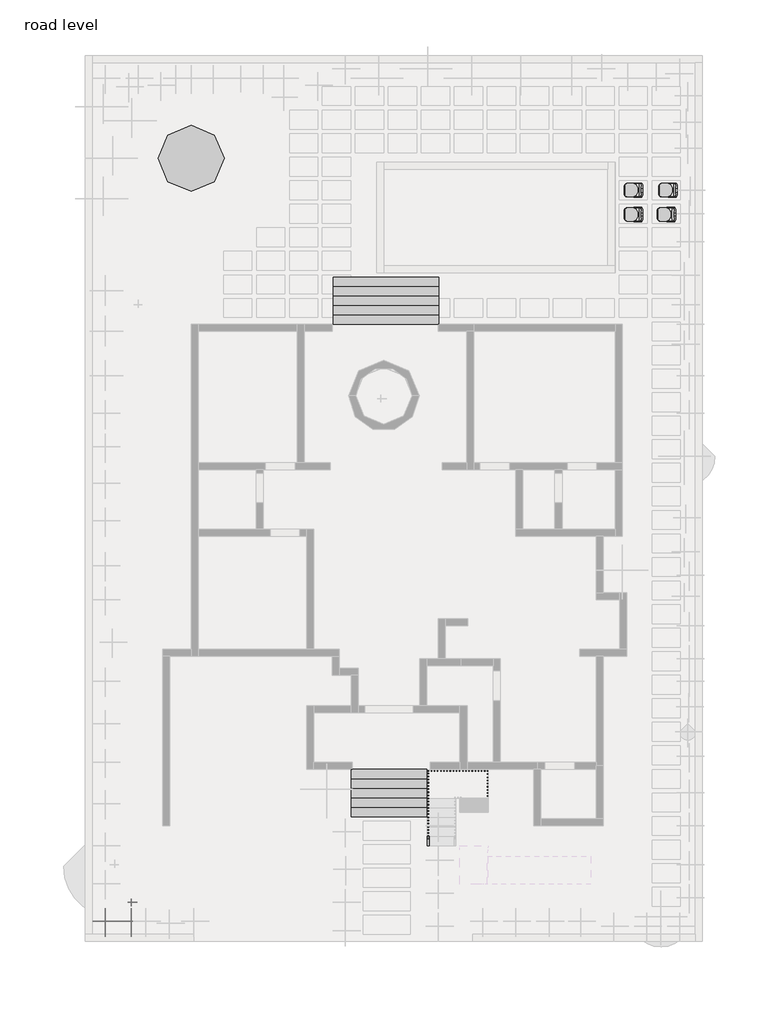
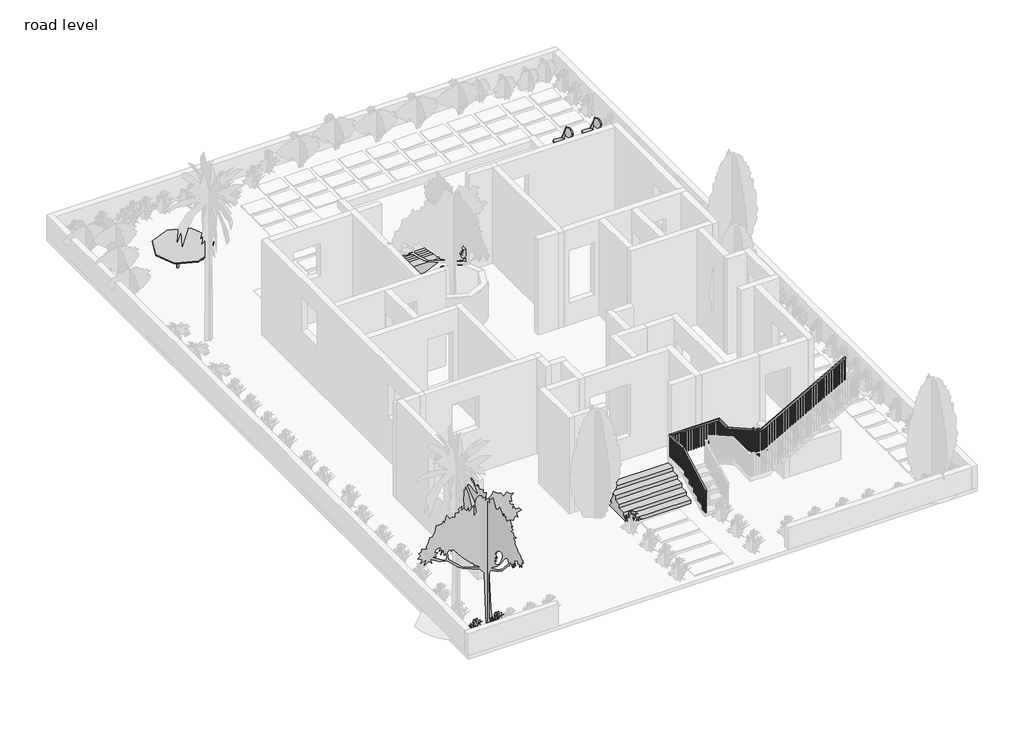
# One storey, part 4 of 5: 7 furniture elements, 3 geographic elements, 1 railing.
"""IFC4 building model written with IfcOpenShell, lengths in millimetres."""

from ifc_helpers import new_model, si_unit, frame, origin, place, context, project, spatial, polyline, outline, extrude, faceted_brep, transform, mapped, element, save
from components import casework_1_casework_1_a8a15752, casework_3_casework_1_715d5e0d, furniture_eb3a3c23, furniture_02b286f5, rpc_plant_tropical_55f6ff97, rpc_tree_tropical_grass_palm_18_ffc4a38a

model = new_model("IFC4")

# Units and contexts
model_context = context("Model", 3, world=origin())
ifc_project = project(units=[si_unit("LENGTHUNIT", "METRE", prefix="MILLI")], contexts=[model_context])

# Site, building, storey
site = spatial("IfcSite", under=ifc_project)
building = spatial("IfcBuilding", under=site)
storey = spatial("IfcBuildingStorey", under=building, Name="road level", Elevation=0.0)

# Furniture
placement = place(None, origin())
casework_1_casework_1_shape = casework_1_casework_1_a8a15752(model_context)
element("IfcFurniture", 1, ObjectType="Casework 1 : Casework 1", at=placement, inside=storey, context=model_context, shape_type="MappedRepresentation", body=[
    mapped(casework_1_casework_1_shape, transform((0.0, 0.0, 0.0), x_axis=(1.0, 0.0, 0.0), y_axis=(0.0, 1.0, 0.0), z_axis=(0.0, 0.0, 1.0))),
])
casework_3_casework_1_shape = casework_3_casework_1_715d5e0d(model_context)
element("IfcFurniture", 2, ObjectType="Casework 3 : Casework 1", at=placement, inside=storey, context=model_context, shape_type="MappedRepresentation", body=[
    mapped(casework_3_casework_1_shape, transform((0.0, 0.0, 0.0), x_axis=(1.0, 0.0, 0.0), y_axis=(0.0, 1.0, 0.0), z_axis=(0.0, 0.0, 1.0))),
])
furniture_shape = furniture_eb3a3c23(model_context)
element("IfcFurniture", 3, ObjectType="Seating-Auditorium : 18\" x 24\" x 30\"", at=placement, inside=storey, context=model_context, shape_type="MappedRepresentation", body=[
    mapped(furniture_shape, transform((13048.714907, 18716.9628198, 50.8), x_axis=(0.0, 1.0, 0.0), y_axis=(-1.0, 0.0, 0.0), z_axis=(0.0, 0.0, 1.0))),
])
element("IfcFurniture", 4, ObjectType="Seating-Auditorium : 18\" x 24\" x 30\"", at=placement, inside=storey, context=model_context, shape_type="MappedRepresentation", body=[
    mapped(furniture_shape, transform((13048.714907, 17929.5628198, 50.8), x_axis=(0.0, 1.0, 0.0), y_axis=(-1.0, 0.0, 0.0), z_axis=(0.0, 0.0, 1.0))),
])
element("IfcFurniture", 5, ObjectType="Seating-Auditorium : 18\" x 24\" x 30\"", at=placement, inside=storey, context=model_context, shape_type="MappedRepresentation", body=[
    mapped(furniture_shape, transform((14115.514907, 17929.5628198, 50.8), x_axis=(0.0, 1.0, 0.0), y_axis=(-1.0, 0.0, 0.0), z_axis=(0.0, 0.0, 1.0))),
])
element("IfcFurniture", 6, ObjectType="Seating-Auditorium : 18\" x 24\" x 30\"", at=placement, inside=storey, context=model_context, shape_type="MappedRepresentation", body=[
    mapped(furniture_shape, transform((14166.314907, 18716.9628198, 50.8), x_axis=(0.0, 1.0, 0.0), y_axis=(-1.0, 0.0, 0.0), z_axis=(0.0, 0.0, 1.0))),
])
furniture_2_shape = furniture_02b286f5(model_context)
element("IfcFurniture", 7, ObjectType="Table-Dining Round : 84\" Diameter", at=placement, inside=storey, context=model_context, shape_type="MappedRepresentation", body=[
    mapped(furniture_2_shape, transform((-1573.2306847, 20091.2693772, 0.0), x_axis=(1.0, 0.0, 0.0), y_axis=(0.0, 1.0, 0.0), z_axis=(0.0, 0.0, 1.0))),
])

# Geographic elements
rpc_plant_tropical_shape = rpc_plant_tropical_55f6ff97(model_context)
element("IfcGeographicElement", 8, ObjectType="RPC Plant - Tropical", at=placement, inside=storey, context=model_context, shape_type="MappedRepresentation", body=[
    mapped(rpc_plant_tropical_shape, transform((-4250.8487175, -4782.4093114, 0.0), x_axis=(1.0, 0.0, 0.0), y_axis=(0.0, 1.0, 0.0), z_axis=(0.0, 0.0, 1.0))),
])
element("IfcGeographicElement", 9, ObjectType="RPC Plant - Tropical", at=placement, inside=storey, context=model_context, shape_type="MappedRepresentation", body=[
    mapped(rpc_plant_tropical_shape, transform((-3412.6487175, -4782.4093114, 0.0), x_axis=(1.0, 0.0, 0.0), y_axis=(0.0, 1.0, 0.0), z_axis=(0.0, 0.0, 1.0))),
])
rpc_tree_tropical_grass_palm_18_shape = rpc_tree_tropical_grass_palm_18_ffc4a38a(model_context)
element("IfcGeographicElement", 10, ObjectType="RPC Tree - Tropical : Grass Palm - 18'", at=placement, inside=storey, context=model_context, shape_type="MappedRepresentation", body=[
    mapped(rpc_tree_tropical_grass_palm_18_shape, transform((-3412.6487175, -4172.8093114, 0.0), x_axis=(1.0, 0.0, 0.0), y_axis=(0.0, 1.0, 0.0), z_axis=(0.0, 0.0, 1.0))),
])

# Railing
element("IfcRailing", 11, ObjectType="Handrail - Rectangular", at=placement, inside=storey, context=model_context, shape_type="SolidModel", body=[
    faceted_brep([(6178.0083823, -2332.334977, 1085.85), (6178.0083823, -2332.334977, 1027.5647478), (6228.8083823, -2332.334977, 1027.5647478), (6228.8083823, -2332.334977, 1085.85), (6178.0083823, -808.334977, 1943.1), (6178.0083823, -795.0278619, 1892.3), (6228.8083823, -795.0278619, 1892.3), (6228.8083823, -808.334977, 1943.1), (6178.0083823, 106.065023, 1943.1), (6178.0083823, 106.065023, 1892.3), (6228.8083823, 55.265023, 1892.3), (6228.8083823, 55.265023, 1943.1), (8143.1297505, 106.065023, 1943.1), (8143.1297505, 106.065023, 1892.3), (8092.3297505, 55.265023, 1892.3), (8092.3297505, 55.265023, 1943.1), (8143.1297505, -503.534977, 1943.1), (8143.1297505, -516.842092, 1892.3), (8092.3297505, -516.842092, 1892.3), (8092.3297505, -503.534977, 1943.1), (8143.1297505, -808.334977, 2114.55), (8143.1297505, -833.2402479, 2070.2739627), (8092.3297505, -833.2402479, 2070.2739627), (8092.3297505, -808.334977, 2114.55), (8143.1297505, -2229.3239999, 2913.8563254), (8143.1297505, -2280.1239999, 2884.1460732), (8092.3297505, -2280.1239999, 2884.1460732), (8092.3297505, -2229.3239999, 2913.8563254), (8143.1297505, -2229.3239999, 2971.8), (8143.1297505, -2280.1239999, 2921.0), (8092.3297505, -2280.1239999, 2921.0), (8092.3297505, -2229.3239999, 2971.8), (8143.1297505, -2332.334977, 2971.8), (8143.1297505, -2332.334977, 2921.0), (8092.3297505, -2329.5130228, 2921.0), (8092.3297505, -2329.5130228, 2971.8), (8131.7203808, -2434.7121604, 2971.8), (8131.7203808, -2434.7121604, 2921.0), (8081.232937, -2429.0856146, 2921.0), (8081.232937, -2429.0856146, 2971.8), (8113.1386293, -2601.4476967, 2971.8), (8107.5120834, -2651.9351405, 2921.0), (8057.0246396, -2646.3085946, 2921.0), (8062.6511855, -2595.8211508, 2971.8), (8113.1386293, -2601.4476967, 3184.4317867), (8107.5120834, -2651.9351405, 3133.6317867), (8057.0246396, -2646.3085946, 3133.6317867), (8062.6511855, -2595.8211508, 3184.4317867), (8105.0297505, -2674.2093114, 3184.4317867), (8105.0297505, -2674.2093114, 3133.6317867), (8048.2538809, -2725.0093114, 3133.6317867), (8048.2538809, -2725.0093114, 3184.4317867), (8178.2418157, -2674.2093114, 3184.4317867), (8191.5489308, -2674.2093114, 3133.6317867), (8191.5489308, -2725.0093114, 3133.6317867), (8178.2418157, -2725.0093114, 3184.4317867), (11457.8297505, -2674.2093114, 5029.2), (11457.8297505, -2725.0093114, 5029.2), (11457.8297505, -2725.0093114, 4970.9147478), (11457.8297505, -2674.2093114, 4970.9147478)], [[[0, 1, 2, 3]], [[1, 0, 4, 5]], [[2, 1, 5, 6]], [[3, 2, 6, 7]], [[0, 3, 7, 4]], [[5, 4, 8, 9]], [[6, 5, 9, 10]], [[7, 6, 10, 11]], [[4, 7, 11, 8]], [[9, 8, 12, 13]], [[10, 9, 13, 14]], [[11, 10, 14, 15]], [[8, 11, 15, 12]], [[13, 12, 16, 17]], [[14, 13, 17, 18]], [[15, 14, 18, 19]], [[12, 15, 19, 16]], [[17, 16, 20, 21]], [[18, 17, 21, 22]], [[19, 18, 22, 23]], [[16, 19, 23, 20]], [[21, 20, 24, 25]], [[22, 21, 25, 26]], [[23, 22, 26, 27]], [[20, 23, 27, 24]], [[25, 24, 28, 29]], [[26, 25, 29, 30]], [[27, 26, 30, 31]], [[24, 27, 31, 28]], [[29, 28, 32, 33]], [[30, 29, 33, 34]], [[31, 30, 34, 35]], [[28, 31, 35, 32]], [[33, 32, 36, 37]], [[34, 33, 37, 38]], [[35, 34, 38, 39]], [[32, 35, 39, 36]], [[37, 36, 40, 41]], [[38, 37, 41, 42]], [[39, 38, 42, 43]], [[36, 39, 43, 40]], [[41, 40, 44, 45]], [[42, 41, 45, 46]], [[43, 42, 46, 47]], [[40, 43, 47, 44]], [[45, 44, 48, 49]], [[46, 45, 49, 50]], [[47, 46, 50, 51]], [[44, 47, 51, 48]], [[49, 48, 52, 53]], [[50, 49, 53, 54]], [[51, 50, 54, 55]], [[48, 51, 55, 52]], [[56, 57, 58, 59]], [[53, 52, 56, 59]], [[54, 53, 59, 58]], [[55, 54, 58, 57]], [[52, 55, 57, 56]]]),
    extrude(outline(polyline([(4949.588722, 11419.9168157), (3943.35, 11419.9168157), (3943.35, 11438.9668157), (4960.304347, 11438.9668157), (4949.588722, 11419.9168157)])), frame((0.0, -2709.1343114, 0.0), z_axis=(0.0, 1.0, 0.0), x_axis=(0.0, 0.0, 1.0)), (0.0, 0.0, 1.0), 19.05),
    extrude(outline(polyline([(4892.438722, 11318.3168157), (3943.35, 11318.3168157), (3943.35, 11337.3668157), (4903.154347, 11337.3668157), (4892.438722, 11318.3168157)])), frame((0.0, -2709.1343114, 0.0), z_axis=(0.0, 1.0, 0.0), x_axis=(0.0, 0.0, 1.0)), (0.0, 0.0, 1.0), 19.05),
    extrude(outline(polyline([(4835.288722, 11216.7168157), (3943.35, 11216.7168157), (3943.35, 11235.7668157), (4846.004347, 11235.7668157), (4835.288722, 11216.7168157)])), frame((0.0, -2709.1343114, 0.0), z_axis=(0.0, 1.0, 0.0), x_axis=(0.0, 0.0, 1.0)), (0.0, 0.0, 1.0), 19.05),
    extrude(outline(polyline([(4778.138722, 11115.1168157), (3771.9, 11115.1168157), (3771.9, 11134.1668157), (4788.854347, 11134.1668157), (4778.138722, 11115.1168157)])), frame((0.0, -2709.1343114, 0.0), z_axis=(0.0, 1.0, 0.0), x_axis=(0.0, 0.0, 1.0)), (0.0, 0.0, 1.0), 19.05),
    extrude(outline(polyline([(4720.988722, 11013.5168157), (3771.9, 11013.5168157), (3771.9, 11032.5668157), (4731.704347, 11032.5668157), (4720.988722, 11013.5168157)])), frame((0.0, -2709.1343114, 0.0), z_axis=(0.0, 1.0, 0.0), x_axis=(0.0, 0.0, 1.0)), (0.0, 0.0, 1.0), 19.05),
    extrude(outline(polyline([(4663.838722, 10911.9168157), (3771.9, 10911.9168157), (3771.9, 10930.9668157), (4674.554347, 10930.9668157), (4663.838722, 10911.9168157)])), frame((0.0, -2709.1343114, 0.0), z_axis=(0.0, 1.0, 0.0), x_axis=(0.0, 0.0, 1.0)), (0.0, 0.0, 1.0), 19.05),
    extrude(outline(polyline([(4606.688722, 10810.3168157), (3600.45, 10810.3168157), (3600.45, 10829.3668157), (4617.404347, 10829.3668157), (4606.688722, 10810.3168157)])), frame((0.0, -2709.1343114, 0.0), z_axis=(0.0, 1.0, 0.0), x_axis=(0.0, 0.0, 1.0)), (0.0, 0.0, 1.0), 19.05),
    extrude(outline(polyline([(4549.538722, 10708.7168157), (3600.45, 10708.7168157), (3600.45, 10727.7668157), (4560.254347, 10727.7668157), (4549.538722, 10708.7168157)])), frame((0.0, -2709.1343114, 0.0), z_axis=(0.0, 1.0, 0.0), x_axis=(0.0, 0.0, 1.0)), (0.0, 0.0, 1.0), 19.05),
    extrude(outline(polyline([(4492.388722, 10607.1168157), (3600.45, 10607.1168157), (3600.45, 10626.1668157), (4503.104347, 10626.1668157), (4492.388722, 10607.1168157)])), frame((0.0, -2709.1343114, 0.0), z_axis=(0.0, 1.0, 0.0), x_axis=(0.0, 0.0, 1.0)), (0.0, 0.0, 1.0), 19.05),
    extrude(outline(polyline([(4435.238722, 10505.5168157), (3429.0, 10505.5168157), (3429.0, 10524.5668157), (4445.954347, 10524.5668157), (4435.238722, 10505.5168157)])), frame((0.0, -2709.1343114, 0.0), z_axis=(0.0, 1.0, 0.0), x_axis=(0.0, 0.0, 1.0)), (0.0, 0.0, 1.0), 19.05),
    extrude(outline(polyline([(4378.088722, 10403.9168157), (3429.0, 10403.9168157), (3429.0, 10422.9668157), (4388.804347, 10422.9668157), (4378.088722, 10403.9168157)])), frame((0.0, -2709.1343114, 0.0), z_axis=(0.0, 1.0, 0.0), x_axis=(0.0, 0.0, 1.0)), (0.0, 0.0, 1.0), 19.05),
    extrude(outline(polyline([(4320.938722, 10302.3168157), (3429.0, 10302.3168157), (3429.0, 10321.3668157), (4331.654347, 10321.3668157), (4320.938722, 10302.3168157)])), frame((0.0, -2709.1343114, 0.0), z_axis=(0.0, 1.0, 0.0), x_axis=(0.0, 0.0, 1.0)), (0.0, 0.0, 1.0), 19.05),
    extrude(outline(polyline([(4263.788722, 10200.7168157), (3257.55, 10200.7168157), (3257.55, 10219.7668157), (4274.504347, 10219.7668157), (4263.788722, 10200.7168157)])), frame((0.0, -2709.1343114, 0.0), z_axis=(0.0, 1.0, 0.0), x_axis=(0.0, 0.0, 1.0)), (0.0, 0.0, 1.0), 19.05),
    extrude(outline(polyline([(4206.638722, 10099.1168157), (3257.55, 10099.1168157), (3257.55, 10118.1668157), (4217.354347, 10118.1668157), (4206.638722, 10099.1168157)])), frame((0.0, -2709.1343114, 0.0), z_axis=(0.0, 1.0, 0.0), x_axis=(0.0, 0.0, 1.0)), (0.0, 0.0, 1.0), 19.05),
    extrude(outline(polyline([(4149.488722, 9997.5168157), (3257.55, 9997.5168157), (3257.55, 10016.5668157), (4160.204347, 10016.5668157), (4149.488722, 9997.5168157)])), frame((0.0, -2709.1343114, 0.0), z_axis=(0.0, 1.0, 0.0), x_axis=(0.0, 0.0, 1.0)), (0.0, 0.0, 1.0), 19.05),
    extrude(outline(polyline([(4092.338722, 9895.9168157), (3086.1, 9895.9168157), (3086.1, 9914.9668157), (4103.054347, 9914.9668157), (4092.338722, 9895.9168157)])), frame((0.0, -2709.1343114, 0.0), z_axis=(0.0, 1.0, 0.0), x_axis=(0.0, 0.0, 1.0)), (0.0, 0.0, 1.0), 19.05),
    extrude(outline(polyline([(4035.188722, 9794.3168157), (3086.1, 9794.3168157), (3086.1, 9813.3668157), (4045.904347, 9813.3668157), (4035.188722, 9794.3168157)])), frame((0.0, -2709.1343114, 0.0), z_axis=(0.0, 1.0, 0.0), x_axis=(0.0, 0.0, 1.0)), (0.0, 0.0, 1.0), 19.05),
    extrude(outline(polyline([(3978.038722, 9692.7168157), (3086.1, 9692.7168157), (3086.1, 9711.7668157), (3988.754347, 9711.7668157), (3978.038722, 9692.7168157)])), frame((0.0, -2709.1343114, 0.0), z_axis=(0.0, 1.0, 0.0), x_axis=(0.0, 0.0, 1.0)), (0.0, 0.0, 1.0), 19.05),
    extrude(outline(polyline([(3920.888722, 9591.1168157), (2914.65, 9591.1168157), (2914.65, 9610.1668157), (3931.604347, 9610.1668157), (3920.888722, 9591.1168157)])), frame((0.0, -2709.1343114, 0.0), z_axis=(0.0, 1.0, 0.0), x_axis=(0.0, 0.0, 1.0)), (0.0, 0.0, 1.0), 19.05),
    extrude(outline(polyline([(3863.738722, 9489.5168157), (2914.65, 9489.5168157), (2914.65, 9508.5668157), (3874.454347, 9508.5668157), (3863.738722, 9489.5168157)])), frame((0.0, -2709.1343114, 0.0), z_axis=(0.0, 1.0, 0.0), x_axis=(0.0, 0.0, 1.0)), (0.0, 0.0, 1.0), 19.05),
    extrude(outline(polyline([(3806.588722, 9387.9168157), (2914.65, 9387.9168157), (2914.65, 9406.9668157), (3817.304347, 9406.9668157), (3806.588722, 9387.9168157)])), frame((0.0, -2709.1343114, 0.0), z_axis=(0.0, 1.0, 0.0), x_axis=(0.0, 0.0, 1.0)), (0.0, 0.0, 1.0), 19.05),
    extrude(outline(polyline([(3749.438722, 9286.3168157), (2743.2, 9286.3168157), (2743.2, 9305.3668157), (3760.154347, 9305.3668157), (3749.438722, 9286.3168157)])), frame((0.0, -2709.1343114, 0.0), z_axis=(0.0, 1.0, 0.0), x_axis=(0.0, 0.0, 1.0)), (0.0, 0.0, 1.0), 19.05),
    extrude(outline(polyline([(3692.288722, 9184.7168157), (2743.2, 9184.7168157), (2743.2, 9203.7668157), (3703.004347, 9203.7668157), (3692.288722, 9184.7168157)])), frame((0.0, -2709.1343114, 0.0), z_axis=(0.0, 1.0, 0.0), x_axis=(0.0, 0.0, 1.0)), (0.0, 0.0, 1.0), 19.05),
    extrude(outline(polyline([(3635.138722, 9083.1168157), (2743.2, 9083.1168157), (2743.2, 9102.1668157), (3645.854347, 9102.1668157), (3635.138722, 9083.1168157)])), frame((0.0, -2709.1343114, 0.0), z_axis=(0.0, 1.0, 0.0), x_axis=(0.0, 0.0, 1.0)), (0.0, 0.0, 1.0), 19.05),
    extrude(outline(polyline([(3577.988722, 8981.5168157), (2571.75, 8981.5168157), (2571.75, 9000.5668157), (3588.704347, 9000.5668157), (3577.988722, 8981.5168157)])), frame((0.0, -2709.1343114, 0.0), z_axis=(0.0, 1.0, 0.0), x_axis=(0.0, 0.0, 1.0)), (0.0, 0.0, 1.0), 19.05),
    extrude(outline(polyline([(3520.838722, 8879.9168157), (2571.75, 8879.9168157), (2571.75, 8898.9668157), (3531.554347, 8898.9668157), (3520.838722, 8879.9168157)])), frame((0.0, -2709.1343114, 0.0), z_axis=(0.0, 1.0, 0.0), x_axis=(0.0, 0.0, 1.0)), (0.0, 0.0, 1.0), 19.05),
    extrude(outline(polyline([(3463.688722, 8778.3168157), (2571.75, 8778.3168157), (2571.75, 8797.3668157), (3474.404347, 8797.3668157), (3463.688722, 8778.3168157)])), frame((0.0, -2709.1343114, 0.0), z_axis=(0.0, 1.0, 0.0), x_axis=(0.0, 0.0, 1.0)), (0.0, 0.0, 1.0), 19.05),
    extrude(outline(polyline([(3406.538722, 8676.7168157), (2400.3, 8676.7168157), (2400.3, 8695.7668157), (3417.254347, 8695.7668157), (3406.538722, 8676.7168157)])), frame((0.0, -2709.1343114, 0.0), z_axis=(0.0, 1.0, 0.0), x_axis=(0.0, 0.0, 1.0)), (0.0, 0.0, 1.0), 19.05),
    extrude(outline(polyline([(3349.388722, 8575.1168157), (2400.3, 8575.1168157), (2400.3, 8594.1668157), (3360.104347, 8594.1668157), (3349.388722, 8575.1168157)])), frame((0.0, -2709.1343114, 0.0), z_axis=(0.0, 1.0, 0.0), x_axis=(0.0, 0.0, 1.0)), (0.0, 0.0, 1.0), 19.05),
    extrude(outline(polyline([(3292.238722, 8473.5168157), (2400.3, 8473.5168157), (2400.3, 8492.5668157), (3302.954347, 8492.5668157), (3292.238722, 8473.5168157)])), frame((0.0, -2709.1343114, 0.0), z_axis=(0.0, 1.0, 0.0), x_axis=(0.0, 0.0, 1.0)), (0.0, 0.0, 1.0), 19.05),
    extrude(outline(polyline([(3235.088722, 8371.9168157), (2228.85, 8371.9168157), (2228.85, 8390.9668157), (3245.804347, 8390.9668157), (3235.088722, 8371.9168157)])), frame((0.0, -2709.1343114, 0.0), z_axis=(0.0, 1.0, 0.0), x_axis=(0.0, 0.0, 1.0)), (0.0, 0.0, 1.0), 19.05),
    extrude(outline(polyline([(3177.938722, 8270.3168157), (2228.85, 8270.3168157), (2228.85, 8289.3668157), (3188.654347, 8289.3668157), (3177.938722, 8270.3168157)])), frame((0.0, -2709.1343114, 0.0), z_axis=(0.0, 1.0, 0.0), x_axis=(0.0, 0.0, 1.0)), (0.0, 0.0, 1.0), 19.05),
    extrude(outline(polyline([(3120.788722, 8168.7168157), (2228.85, 8168.7168157), (2228.85, 8187.7668157), (3131.504347, 8187.7668157), (3120.788722, 8168.7168157)])), frame((0.0, -2709.1343114, 0.0), z_axis=(0.0, 1.0, 0.0), x_axis=(0.0, 0.0, 1.0)), (0.0, 0.0, 1.0), 19.05),
    extrude(outline(polyline([(8094.4918486, -2625.4372443), (8092.381894, -2644.3700358), (8073.4491025, -2642.2600811), (8075.5590572, -2623.3272896), (8094.4918486, -2625.4372443)])), frame((0.0, 0.0, 2057.4), z_axis=(0.0, 0.0, 1.0), x_axis=(1.0, 0.0, 0.0)), (0.0, 0.0, 1.0), 1076.2317867),
    extrude(outline(polyline([(8105.7449403, -2524.4623567), (8103.6349856, -2543.3951481), (8084.7021942, -2541.2851935), (8086.8121489, -2522.352402), (8105.7449403, -2524.4623567)])), frame((0.0, 0.0, 2057.4), z_axis=(0.0, 0.0, 1.0), x_axis=(1.0, 0.0, 0.0)), (0.0, 0.0, 1.0), 863.6),
    extrude(outline(polyline([(8116.9980319, -2423.4874691), (8114.8880773, -2442.4202605), (8095.9552858, -2440.3103059), (8098.0652405, -2421.3775144), (8116.9980319, -2423.4874691)])), frame((0.0, 0.0, 2057.4), z_axis=(0.0, 0.0, 1.0), x_axis=(1.0, 0.0, 0.0)), (0.0, 0.0, 1.0), 863.6),
    extrude(outline(polyline([(8127.2547505, -2221.209977), (8127.2547505, -2240.259977), (8108.2047505, -2240.259977), (8108.2047505, -2221.209977), (8127.2547505, -2221.209977)])), frame((0.0, 0.0, 1885.95), z_axis=(0.0, 0.0, 1.0), x_axis=(1.0, 0.0, 0.0)), (0.0, 0.0, 1.0), 1035.05),
    extrude(outline(polyline([(-2119.609977, 2793.8569353), (-2119.609977, 1885.95), (-2138.659977, 1885.95), (-2138.659977, 2804.5725603), (-2119.609977, 2793.8569353)])), frame((8108.2047505, 0.0, 0.0), z_axis=(1.0, 0.0, 0.0), x_axis=(0.0, 1.0, 0.0)), (0.0, 0.0, 1.0), 19.05),
    extrude(outline(polyline([(-2018.009977, 2736.7069353), (-2018.009977, 1885.95), (-2037.059977, 1885.95), (-2037.059977, 2747.4225603), (-2018.009977, 2736.7069353)])), frame((8108.2047505, 0.0, 0.0), z_axis=(1.0, 0.0, 0.0), x_axis=(0.0, 1.0, 0.0)), (0.0, 0.0, 1.0), 19.05),
    extrude(outline(polyline([(-1916.409977, 2679.5569353), (-1916.409977, 1714.5), (-1935.459977, 1714.5), (-1935.459977, 2690.2725603), (-1916.409977, 2679.5569353)])), frame((8108.2047505, 0.0, 0.0), z_axis=(1.0, 0.0, 0.0), x_axis=(0.0, 1.0, 0.0)), (0.0, 0.0, 1.0), 19.05),
    extrude(outline(polyline([(-1814.809977, 2622.4069353), (-1814.809977, 1714.5), (-1833.859977, 1714.5), (-1833.859977, 2633.1225603), (-1814.809977, 2622.4069353)])), frame((8108.2047505, 0.0, 0.0), z_axis=(1.0, 0.0, 0.0), x_axis=(0.0, 1.0, 0.0)), (0.0, 0.0, 1.0), 19.05),
    extrude(outline(polyline([(-1713.209977, 2565.2569353), (-1713.209977, 1714.5), (-1732.259977, 1714.5), (-1732.259977, 2575.9725603), (-1713.209977, 2565.2569353)])), frame((8108.2047505, 0.0, 0.0), z_axis=(1.0, 0.0, 0.0), x_axis=(0.0, 1.0, 0.0)), (0.0, 0.0, 1.0), 19.05),
    extrude(outline(polyline([(-1611.609977, 2508.1069353), (-1611.609977, 1543.05), (-1630.659977, 1543.05), (-1630.659977, 2518.8225603), (-1611.609977, 2508.1069353)])), frame((8108.2047505, 0.0, 0.0), z_axis=(1.0, 0.0, 0.0), x_axis=(0.0, 1.0, 0.0)), (0.0, 0.0, 1.0), 19.05),
    extrude(outline(polyline([(-1510.009977, 2450.9569353), (-1510.009977, 1543.05), (-1529.059977, 1543.05), (-1529.059977, 2461.6725603), (-1510.009977, 2450.9569353)])), frame((8108.2047505, 0.0, 0.0), z_axis=(1.0, 0.0, 0.0), x_axis=(0.0, 1.0, 0.0)), (0.0, 0.0, 1.0), 19.05),
    extrude(outline(polyline([(-1408.409977, 2393.8069353), (-1408.409977, 1543.05), (-1427.459977, 1543.05), (-1427.459977, 2404.5225603), (-1408.409977, 2393.8069353)])), frame((8108.2047505, 0.0, 0.0), z_axis=(1.0, 0.0, 0.0), x_axis=(0.0, 1.0, 0.0)), (0.0, 0.0, 1.0), 19.05),
    extrude(outline(polyline([(-1306.809977, 2336.6569353), (-1306.809977, 1371.6), (-1325.859977, 1371.6), (-1325.859977, 2347.3725603), (-1306.809977, 2336.6569353)])), frame((8108.2047505, 0.0, 0.0), z_axis=(1.0, 0.0, 0.0), x_axis=(0.0, 1.0, 0.0)), (0.0, 0.0, 1.0), 19.05),
    extrude(outline(polyline([(-1205.209977, 2279.5069353), (-1205.209977, 1371.6), (-1224.259977, 1371.6), (-1224.259977, 2290.2225603), (-1205.209977, 2279.5069353)])), frame((8108.2047505, 0.0, 0.0), z_axis=(1.0, 0.0, 0.0), x_axis=(0.0, 1.0, 0.0)), (0.0, 0.0, 1.0), 19.05),
    extrude(outline(polyline([(-1103.609977, 2222.3569353), (-1103.609977, 1371.6), (-1122.659977, 1371.6), (-1122.659977, 2233.0725603), (-1103.609977, 2222.3569353)])), frame((8108.2047505, 0.0, 0.0), z_axis=(1.0, 0.0, 0.0), x_axis=(0.0, 1.0, 0.0)), (0.0, 0.0, 1.0), 19.05),
    extrude(outline(polyline([(-1002.009977, 2165.2069353), (-1002.009977, 1200.15), (-1021.059977, 1200.15), (-1021.059977, 2175.9225603), (-1002.009977, 2165.2069353)])), frame((8108.2047505, 0.0, 0.0), z_axis=(1.0, 0.0, 0.0), x_axis=(0.0, 1.0, 0.0)), (0.0, 0.0, 1.0), 19.05),
    extrude(outline(polyline([(-900.409977, 2108.0569353), (-900.409977, 1200.15), (-919.459977, 1200.15), (-919.459977, 2118.7725603), (-900.409977, 2108.0569353)])), frame((8108.2047505, 0.0, 0.0), z_axis=(1.0, 0.0, 0.0), x_axis=(0.0, 1.0, 0.0)), (0.0, 0.0, 1.0), 19.05),
    extrude(outline(polyline([(-722.609977, 2008.0444353), (-722.609977, 1028.7), (-741.659977, 1028.7), (-741.659977, 2018.7600603), (-722.609977, 2008.0444353)])), frame((8108.2047505, 0.0, 0.0), z_axis=(1.0, 0.0, 0.0), x_axis=(0.0, 1.0, 0.0)), (0.0, 0.0, 1.0), 19.05),
    extrude(outline(polyline([(-621.009977, 1950.8944353), (-621.009977, 1028.7), (-640.059977, 1028.7), (-640.059977, 1961.6100603), (-621.009977, 1950.8944353)])), frame((8108.2047505, 0.0, 0.0), z_axis=(1.0, 0.0, 0.0), x_axis=(0.0, 1.0, 0.0)), (0.0, 0.0, 1.0), 19.05),
    extrude(outline(polyline([(-519.409977, 1893.7444353), (-519.409977, 1028.7), (-538.459977, 1028.7), (-538.459977, 1904.4600603), (-519.409977, 1893.7444353)])), frame((8108.2047505, 0.0, 0.0), z_axis=(1.0, 0.0, 0.0), x_axis=(0.0, 1.0, 0.0)), (0.0, 0.0, 1.0), 19.05),
    extrude(outline(polyline([(8127.2547505, -417.809977), (8127.2547505, -436.859977), (8108.2047505, -436.859977), (8108.2047505, -417.809977), (8127.2547505, -417.809977)])), frame((0.0, 0.0, 1028.7), z_axis=(0.0, 0.0, 1.0), x_axis=(1.0, 0.0, 0.0)), (0.0, 0.0, 1.0), 863.6),
    extrude(outline(polyline([(8127.2547505, -316.209977), (8127.2547505, -335.259977), (8108.2047505, -335.259977), (8108.2047505, -316.209977), (8127.2547505, -316.209977)])), frame((0.0, 0.0, 1028.7), z_axis=(0.0, 0.0, 1.0), x_axis=(1.0, 0.0, 0.0)), (0.0, 0.0, 1.0), 863.6),
    extrude(outline(polyline([(8127.2547505, -214.609977), (8127.2547505, -233.659977), (8108.2047505, -233.659977), (8108.2047505, -214.609977), (8127.2547505, -214.609977)])), frame((0.0, 0.0, 1028.7), z_axis=(0.0, 0.0, 1.0), x_axis=(1.0, 0.0, 0.0)), (0.0, 0.0, 1.0), 863.6),
    extrude(outline(polyline([(8127.2547505, -113.009977), (8127.2547505, -132.059977), (8108.2047505, -132.059977), (8108.2047505, -113.009977), (8127.2547505, -113.009977)])), frame((0.0, 0.0, 1028.7), z_axis=(0.0, 0.0, 1.0), x_axis=(1.0, 0.0, 0.0)), (0.0, 0.0, 1.0), 863.6),
    extrude(outline(polyline([(8127.2547505, -11.409977), (8127.2547505, -30.459977), (8108.2047505, -30.459977), (8108.2047505, -11.409977), (8127.2547505, -11.409977)])), frame((0.0, 0.0, 1028.7), z_axis=(0.0, 0.0, 1.0), x_axis=(1.0, 0.0, 0.0)), (0.0, 0.0, 1.0), 863.6),
    extrude(outline(polyline([(8022.6833823, 90.190023), (8041.7333823, 90.190023), (8041.7333823, 71.140023), (8022.6833823, 71.140023), (8022.6833823, 90.190023)])), frame((0.0, 0.0, 1028.7), z_axis=(0.0, 0.0, 1.0), x_axis=(1.0, 0.0, 0.0)), (0.0, 0.0, 1.0), 863.6),
    extrude(outline(polyline([(7921.0833823, 90.190023), (7940.1333823, 90.190023), (7940.1333823, 71.140023), (7921.0833823, 71.140023), (7921.0833823, 90.190023)])), frame((0.0, 0.0, 1028.7), z_axis=(0.0, 0.0, 1.0), x_axis=(1.0, 0.0, 0.0)), (0.0, 0.0, 1.0), 863.6),
    extrude(outline(polyline([(7819.4833823, 90.190023), (7838.5333823, 90.190023), (7838.5333823, 71.140023), (7819.4833823, 71.140023), (7819.4833823, 90.190023)])), frame((0.0, 0.0, 1028.7), z_axis=(0.0, 0.0, 1.0), x_axis=(1.0, 0.0, 0.0)), (0.0, 0.0, 1.0), 863.6),
    extrude(outline(polyline([(7717.8833823, 90.190023), (7736.9333823, 90.190023), (7736.9333823, 71.140023), (7717.8833823, 71.140023), (7717.8833823, 90.190023)])), frame((0.0, 0.0, 1028.7), z_axis=(0.0, 0.0, 1.0), x_axis=(1.0, 0.0, 0.0)), (0.0, 0.0, 1.0), 863.6),
    extrude(outline(polyline([(7616.2833823, 90.190023), (7635.3333823, 90.190023), (7635.3333823, 71.140023), (7616.2833823, 71.140023), (7616.2833823, 90.190023)])), frame((0.0, 0.0, 1028.7), z_axis=(0.0, 0.0, 1.0), x_axis=(1.0, 0.0, 0.0)), (0.0, 0.0, 1.0), 863.6),
    extrude(outline(polyline([(7514.6833823, 90.190023), (7533.7333823, 90.190023), (7533.7333823, 71.140023), (7514.6833823, 71.140023), (7514.6833823, 90.190023)])), frame((0.0, 0.0, 1028.7), z_axis=(0.0, 0.0, 1.0), x_axis=(1.0, 0.0, 0.0)), (0.0, 0.0, 1.0), 863.6),
    extrude(outline(polyline([(7413.0833823, 90.190023), (7432.1333823, 90.190023), (7432.1333823, 71.140023), (7413.0833823, 71.140023), (7413.0833823, 90.190023)])), frame((0.0, 0.0, 1028.7), z_axis=(0.0, 0.0, 1.0), x_axis=(1.0, 0.0, 0.0)), (0.0, 0.0, 1.0), 863.6),
    extrude(outline(polyline([(7311.4833823, 90.190023), (7330.5333823, 90.190023), (7330.5333823, 71.140023), (7311.4833823, 71.140023), (7311.4833823, 90.190023)])), frame((0.0, 0.0, 1028.7), z_axis=(0.0, 0.0, 1.0), x_axis=(1.0, 0.0, 0.0)), (0.0, 0.0, 1.0), 863.6),
    extrude(outline(polyline([(7209.8833823, 90.190023), (7228.9333823, 90.190023), (7228.9333823, 71.140023), (7209.8833823, 71.140023), (7209.8833823, 90.190023)])), frame((0.0, 0.0, 1028.7), z_axis=(0.0, 0.0, 1.0), x_axis=(1.0, 0.0, 0.0)), (0.0, 0.0, 1.0), 863.6),
    extrude(outline(polyline([(7108.2833823, 90.190023), (7127.3333823, 90.190023), (7127.3333823, 71.140023), (7108.2833823, 71.140023), (7108.2833823, 90.190023)])), frame((0.0, 0.0, 1028.7), z_axis=(0.0, 0.0, 1.0), x_axis=(1.0, 0.0, 0.0)), (0.0, 0.0, 1.0), 863.6),
    extrude(outline(polyline([(7006.6833823, 90.190023), (7025.7333823, 90.190023), (7025.7333823, 71.140023), (7006.6833823, 71.140023), (7006.6833823, 90.190023)])), frame((0.0, 0.0, 1028.7), z_axis=(0.0, 0.0, 1.0), x_axis=(1.0, 0.0, 0.0)), (0.0, 0.0, 1.0), 863.6),
    extrude(outline(polyline([(6905.0833823, 90.190023), (6924.1333823, 90.190023), (6924.1333823, 71.140023), (6905.0833823, 71.140023), (6905.0833823, 90.190023)])), frame((0.0, 0.0, 1028.7), z_axis=(0.0, 0.0, 1.0), x_axis=(1.0, 0.0, 0.0)), (0.0, 0.0, 1.0), 863.6),
    extrude(outline(polyline([(6803.4833823, 90.190023), (6822.5333823, 90.190023), (6822.5333823, 71.140023), (6803.4833823, 71.140023), (6803.4833823, 90.190023)])), frame((0.0, 0.0, 1028.7), z_axis=(0.0, 0.0, 1.0), x_axis=(1.0, 0.0, 0.0)), (0.0, 0.0, 1.0), 863.6),
    extrude(outline(polyline([(6701.8833823, 90.190023), (6720.9333823, 90.190023), (6720.9333823, 71.140023), (6701.8833823, 71.140023), (6701.8833823, 90.190023)])), frame((0.0, 0.0, 1028.7), z_axis=(0.0, 0.0, 1.0), x_axis=(1.0, 0.0, 0.0)), (0.0, 0.0, 1.0), 863.6),
    extrude(outline(polyline([(6600.2833823, 90.190023), (6619.3333823, 90.190023), (6619.3333823, 71.140023), (6600.2833823, 71.140023), (6600.2833823, 90.190023)])), frame((0.0, 0.0, 1028.7), z_axis=(0.0, 0.0, 1.0), x_axis=(1.0, 0.0, 0.0)), (0.0, 0.0, 1.0), 863.6),
    extrude(outline(polyline([(6498.6833823, 90.190023), (6517.7333823, 90.190023), (6517.7333823, 71.140023), (6498.6833823, 71.140023), (6498.6833823, 90.190023)])), frame((0.0, 0.0, 1028.7), z_axis=(0.0, 0.0, 1.0), x_axis=(1.0, 0.0, 0.0)), (0.0, 0.0, 1.0), 863.6),
    extrude(outline(polyline([(6397.0833823, 90.190023), (6416.1333823, 90.190023), (6416.1333823, 71.140023), (6397.0833823, 71.140023), (6397.0833823, 90.190023)])), frame((0.0, 0.0, 1028.7), z_axis=(0.0, 0.0, 1.0), x_axis=(1.0, 0.0, 0.0)), (0.0, 0.0, 1.0), 863.6),
    extrude(outline(polyline([(6295.4833823, 90.190023), (6314.5333823, 90.190023), (6314.5333823, 71.140023), (6295.4833823, 71.140023), (6295.4833823, 90.190023)])), frame((0.0, 0.0, 1028.7), z_axis=(0.0, 0.0, 1.0), x_axis=(1.0, 0.0, 0.0)), (0.0, 0.0, 1.0), 863.6),
    extrude(outline(polyline([(6193.8833823, -5.059977), (6193.8833823, 13.990023), (6212.9333823, 13.990023), (6212.9333823, -5.059977), (6193.8833823, -5.059977)])), frame((0.0, 0.0, 1028.7), z_axis=(0.0, 0.0, 1.0), x_axis=(1.0, 0.0, 0.0)), (0.0, 0.0, 1.0), 863.6),
    extrude(outline(polyline([(6193.8833823, -106.659977), (6193.8833823, -87.609977), (6212.9333823, -87.609977), (6212.9333823, -106.659977), (6193.8833823, -106.659977)])), frame((0.0, 0.0, 1028.7), z_axis=(0.0, 0.0, 1.0), x_axis=(1.0, 0.0, 0.0)), (0.0, 0.0, 1.0), 863.6),
    extrude(outline(polyline([(6193.8833823, -208.259977), (6193.8833823, -189.209977), (6212.9333823, -189.209977), (6212.9333823, -208.259977), (6193.8833823, -208.259977)])), frame((0.0, 0.0, 1028.7), z_axis=(0.0, 0.0, 1.0), x_axis=(1.0, 0.0, 0.0)), (0.0, 0.0, 1.0), 863.6),
    extrude(outline(polyline([(6193.8833823, -309.859977), (6193.8833823, -290.809977), (6212.9333823, -290.809977), (6212.9333823, -309.859977), (6193.8833823, -309.859977)])), frame((0.0, 0.0, 1028.7), z_axis=(0.0, 0.0, 1.0), x_axis=(1.0, 0.0, 0.0)), (0.0, 0.0, 1.0), 863.6),
    extrude(outline(polyline([(6193.8833823, -411.459977), (6193.8833823, -392.409977), (6212.9333823, -392.409977), (6212.9333823, -411.459977), (6193.8833823, -411.459977)])), frame((0.0, 0.0, 1028.7), z_axis=(0.0, 0.0, 1.0), x_axis=(1.0, 0.0, 0.0)), (0.0, 0.0, 1.0), 863.6),
    extrude(outline(polyline([(6193.8833823, -513.059977), (6193.8833823, -494.009977), (6212.9333823, -494.009977), (6212.9333823, -513.059977), (6193.8833823, -513.059977)])), frame((0.0, 0.0, 1028.7), z_axis=(0.0, 0.0, 1.0), x_axis=(1.0, 0.0, 0.0)), (0.0, 0.0, 1.0), 863.6),
    extrude(outline(polyline([(6193.8833823, -614.659977), (6193.8833823, -595.609977), (6212.9333823, -595.609977), (6212.9333823, -614.659977), (6193.8833823, -614.659977)])), frame((0.0, 0.0, 1028.7), z_axis=(0.0, 0.0, 1.0), x_axis=(1.0, 0.0, 0.0)), (0.0, 0.0, 1.0), 863.6),
    extrude(outline(polyline([(6193.8833823, -716.259977), (6193.8833823, -697.209977), (6212.9333823, -697.209977), (6212.9333823, -716.259977), (6193.8833823, -716.259977)])), frame((0.0, 0.0, 1028.7), z_axis=(0.0, 0.0, 1.0), x_axis=(1.0, 0.0, 0.0)), (0.0, 0.0, 1.0), 863.6),
    extrude(outline(polyline([(-900.409977, 1833.0225603), (-900.409977, 857.25), (-919.459977, 857.25), (-919.459977, 1822.3069353), (-900.409977, 1833.0225603)])), frame((6193.8833823, 0.0, 0.0), z_axis=(1.0, 0.0, 0.0), x_axis=(0.0, 1.0, 0.0)), (0.0, 0.0, 1.0), 19.05),
    extrude(outline(polyline([(-1002.009977, 1775.8725603), (-1002.009977, 857.25), (-1021.059977, 857.25), (-1021.059977, 1765.1569353), (-1002.009977, 1775.8725603)])), frame((6193.8833823, 0.0, 0.0), z_axis=(1.0, 0.0, 0.0), x_axis=(0.0, 1.0, 0.0)), (0.0, 0.0, 1.0), 19.05),
    extrude(outline(polyline([(-1103.609977, 1718.7225603), (-1103.609977, 857.25), (-1122.659977, 857.25), (-1122.659977, 1708.0069353), (-1103.609977, 1718.7225603)])), frame((6193.8833823, 0.0, 0.0), z_axis=(1.0, 0.0, 0.0), x_axis=(0.0, 1.0, 0.0)), (0.0, 0.0, 1.0), 19.05),
    extrude(outline(polyline([(-1205.209977, 1661.5725603), (-1205.209977, 685.8), (-1224.259977, 685.8), (-1224.259977, 1650.8569353), (-1205.209977, 1661.5725603)])), frame((6193.8833823, 0.0, 0.0), z_axis=(1.0, 0.0, 0.0), x_axis=(0.0, 1.0, 0.0)), (0.0, 0.0, 1.0), 19.05),
    extrude(outline(polyline([(-1306.809977, 1604.4225603), (-1306.809977, 685.8), (-1325.859977, 685.8), (-1325.859977, 1593.7069353), (-1306.809977, 1604.4225603)])), frame((6193.8833823, 0.0, 0.0), z_axis=(1.0, 0.0, 0.0), x_axis=(0.0, 1.0, 0.0)), (0.0, 0.0, 1.0), 19.05),
    extrude(outline(polyline([(-1408.409977, 1547.2725603), (-1408.409977, 685.8), (-1427.459977, 685.8), (-1427.459977, 1536.5569353), (-1408.409977, 1547.2725603)])), frame((6193.8833823, 0.0, 0.0), z_axis=(1.0, 0.0, 0.0), x_axis=(0.0, 1.0, 0.0)), (0.0, 0.0, 1.0), 19.05),
    extrude(outline(polyline([(-1510.009977, 1490.1225603), (-1510.009977, 514.35), (-1529.059977, 514.35), (-1529.059977, 1479.4069353), (-1510.009977, 1490.1225603)])), frame((6193.8833823, 0.0, 0.0), z_axis=(1.0, 0.0, 0.0), x_axis=(0.0, 1.0, 0.0)), (0.0, 0.0, 1.0), 19.05),
    extrude(outline(polyline([(-1611.609977, 1432.9725603), (-1611.609977, 514.35), (-1630.659977, 514.35), (-1630.659977, 1422.2569353), (-1611.609977, 1432.9725603)])), frame((6193.8833823, 0.0, 0.0), z_axis=(1.0, 0.0, 0.0), x_axis=(0.0, 1.0, 0.0)), (0.0, 0.0, 1.0), 19.05),
    extrude(outline(polyline([(-1713.209977, 1375.8225603), (-1713.209977, 514.35), (-1732.259977, 514.35), (-1732.259977, 1365.1069353), (-1713.209977, 1375.8225603)])), frame((6193.8833823, 0.0, 0.0), z_axis=(1.0, 0.0, 0.0), x_axis=(0.0, 1.0, 0.0)), (0.0, 0.0, 1.0), 19.05),
    extrude(outline(polyline([(-1814.809977, 1318.6725603), (-1814.809977, 342.9), (-1833.859977, 342.9), (-1833.859977, 1307.9569353), (-1814.809977, 1318.6725603)])), frame((6193.8833823, 0.0, 0.0), z_axis=(1.0, 0.0, 0.0), x_axis=(0.0, 1.0, 0.0)), (0.0, 0.0, 1.0), 19.05),
    extrude(outline(polyline([(-1916.409977, 1261.5225603), (-1916.409977, 342.9), (-1935.459977, 342.9), (-1935.459977, 1250.8069353), (-1916.409977, 1261.5225603)])), frame((6193.8833823, 0.0, 0.0), z_axis=(1.0, 0.0, 0.0), x_axis=(0.0, 1.0, 0.0)), (0.0, 0.0, 1.0), 19.05),
    extrude(outline(polyline([(-2018.009977, 1204.3725603), (-2018.009977, 342.9), (-2037.059977, 342.9), (-2037.059977, 1193.6569353), (-2018.009977, 1204.3725603)])), frame((6193.8833823, 0.0, 0.0), z_axis=(1.0, 0.0, 0.0), x_axis=(0.0, 1.0, 0.0)), (0.0, 0.0, 1.0), 19.05),
    extrude(outline(polyline([(-2119.609977, 1147.2225603), (-2119.609977, 171.45), (-2138.659977, 171.45), (-2138.659977, 1136.5069353), (-2119.609977, 1147.2225603)])), frame((6193.8833823, 0.0, 0.0), z_axis=(1.0, 0.0, 0.0), x_axis=(0.0, 1.0, 0.0)), (0.0, 0.0, 1.0), 19.05),
    extrude(outline(polyline([(-2221.209977, 1090.0725603), (-2221.209977, 171.45), (-2240.259977, 171.45), (-2240.259977, 1079.3569353), (-2221.209977, 1090.0725603)])), frame((6193.8833823, 0.0, 0.0), z_axis=(1.0, 0.0, 0.0), x_axis=(0.0, 1.0, 0.0)), (0.0, 0.0, 1.0), 19.05),
    extrude(outline(polyline([(8087.1631888, -2691.197893), (8085.0532341, -2710.1306844), (8066.1204427, -2708.0207297), (8068.2303973, -2689.0879383), (8087.1631888, -2691.197893)])), frame((0.0, 0.0, 2057.4), z_axis=(0.0, 0.0, 1.0), x_axis=(1.0, 0.0, 0.0)), (0.0, 0.0, 1.0), 1076.2317867),
    extrude(outline(polyline([(8127.2547505, -2321.3989999), (8127.2547505, -2340.4489999), (8108.2047505, -2340.4489999), (8108.2047505, -2321.3989999), (8127.2547505, -2321.3989999)])), frame((0.0, 0.0, 1885.95), z_axis=(0.0, 0.0, 1.0), x_axis=(1.0, 0.0, 0.0)), (0.0, 0.0, 1.0), 1035.05),
    extrude(outline(polyline([(-798.809977, 2050.9069353), (-798.809977, 1028.7), (-817.859977, 1028.7), (-817.859977, 2061.6225603), (-798.809977, 2050.9069353)])), frame((8108.2047505, 0.0, 0.0), z_axis=(1.0, 0.0, 0.0), x_axis=(0.0, 1.0, 0.0)), (0.0, 0.0, 1.0), 19.05),
    extrude(outline(polyline([(8108.2047505, 90.190023), (8127.2547505, 90.190023), (8127.2547505, 71.140023), (8108.2047505, 71.140023), (8108.2047505, 90.190023)])), frame((0.0, 0.0, 1028.7), z_axis=(0.0, 0.0, 1.0), x_axis=(1.0, 0.0, 0.0)), (0.0, 0.0, 1.0), 863.6),
    extrude(outline(polyline([(6193.8833823, 71.140023), (6193.8833823, 90.190023), (6212.9333823, 90.190023), (6212.9333823, 71.140023), (6193.8833823, 71.140023)])), frame((0.0, 0.0, 1028.7), z_axis=(0.0, 0.0, 1.0), x_axis=(1.0, 0.0, 0.0)), (0.0, 0.0, 1.0), 863.6),
    extrude(outline(polyline([(-798.809977, 1890.1725603), (-798.809977, 1028.7), (-817.859977, 1028.7), (-817.859977, 1879.4569353), (-798.809977, 1890.1725603)])), frame((6193.8833823, 0.0, 0.0), z_axis=(1.0, 0.0, 0.0), x_axis=(0.0, 1.0, 0.0)), (0.0, 0.0, 1.0), 19.05),
    extrude(outline(polyline([(4960.1991228, 11438.7797505), (3943.35, 11438.7797505), (3943.35, 11457.8297505), (4970.9147478, 11457.8297505), (4960.1991228, 11438.7797505)])), frame((0.0, -2709.1343114, 0.0), z_axis=(0.0, 1.0, 0.0), x_axis=(0.0, 0.0, 1.0)), (0.0, 0.0, 1.0), 19.05),
    extrude(outline(polyline([(-2313.284977, 1038.2803728), (-2313.284977, 171.45), (-2332.334977, 171.45), (-2332.334977, 1027.5647478), (-2313.284977, 1038.2803728)])), frame((6193.8833823, 0.0, 0.0), z_axis=(1.0, 0.0, 0.0), x_axis=(0.0, 1.0, 0.0)), (0.0, 0.0, 1.0), 19.05),
])

save(model, "model.ifc")

# Revit data of these elements
# Type "Seating-Auditorium : 18\" x 24\" x 30\""
#   Assembly Code = "E2020200"
#   Seat Material = Linen, Beige
#   Frame Material = Steel, Paint Finish, Dark Gray, Matte
#   Default Elevation = 0
# Type "Table-Dining Round : 84\" Diameter"
#   Assembly Code = "E2020200"
#   Diameter = 7' - 0"
#   Height = 1' - 6"
#   Base Material = Pine
#   Top Material = Laminate, Linen, Matte
#   Default Elevation = 0
# Type "RPC Plant - Tropical"
#   built-in parameter 1005198 = "{2, 15},{39, RPC-16-FWM5-GM7X-C67P-4000-ST1L-LVER-AU},{1, 0},{1, 0},{2, 35},{1, 8},{5, Color},{1, 0},{1, 0},{3, 0.8},{3, 0.8},{3, 0.8},{1, 8},{7, BBoxMin},{1, 0},{1, 0},{1, 0},{1, 0},{1, 0},{1, 8},{7, BBoxMax},{1, 0},{1, 0},{1, 0},{1, 0},{1, 0},{2, 11},{9, RPCTypeId},{1, 0},{1, 0},{39, RPC-16-FWM5-GM7X-C67P-4000-ST1L-LVER-AU},{1, 6},{14, RPCPlantHeight},{1, 0},{1, 0},{1, 3},{2, 11},{7, keyword},{1, 0},{1, 0},{99, :Geometry:RPC:Crane Lily:strelitzia:reinae:crane lily:plants:shrub:flower:tropical:bird-of-paradise},{2, 11},{8, category},{1, 0},{1, 0},{17, :Shrubs [General]},{2, 11},{12, LocalizedUID},{1, 0},{1, 0},{10, Crane Lily},{2, 14},{6, Height},{1, 0},{1, 0},{1, 3},{1, 2},{16, Cast Reflections},{1, 0},{1, 0},{1, 0},{1, 2},{12, Cast Shadows},{1, 0},{1, 0},{1, 1},{1, 2},{9, Lock View},{1, 0},{1, 0},{1, 0},{1, 4},{5, ViewC},{1, 0},{1, 0},{1, 0},{2, 11},{20, AdvancedUIDefinition},{1, 0},{1, 0},{0, },{2, 11},{10, AssetLibID},{1, 0},{1, 0},{36, 4D3F6E72-3F99-4203-98E9-AF80B3C7A7A4},{2, 11},{10, BaseSchema},{1, 0},{1, 0},{9, RPCSchema},{2, 11},{12, ExchangeGUID},{1, 0},{1, 0},{0, },{1, 2},{6, Hidden},{1, 0},{1, 0},{1, 0},{1, 4},{11, RPCCategory},{1, 0},{1, 0},{1, 0},{2, 11},{8, RPCImage},{1, 0},{1, 0},{0, },{1, 4},{13, SchemaVersion},{1, 0},{1, 0},{1, 4},{2, 11},{12, UIDefinition},{1, 0},{1, 0},{0, },{2, 11},{6, UIName},{1, 0},{1, 0},{39, RPC-16-FWM5-GM7X-C67P-4000-ST1L-LVER-AU},{2, 11},{11, VersionGUID},{1, 0},{1, 0},{9, RPCSchema},{2, 11},{9, assettype},{1, 0},{1, 0},{11, RPCGeometry},{2, 11},{11, description},{1, 0},{1, 0},{0, },{2, 11},{9, localname},{1, 0},{1, 0},{3, RPC},{2, 11},{9, localtype},{1, 0},{1, 0},{3, RPC},{1, 4},{8, revision},{1, 0},{1, 0},{1, 1},{2, 11},{9, thumbnail},{1, 0},{1, 0},{0, },{1, 4},{7, version},{1, 0},{1, 0},{1, 1},{1, 2},{20, RPC_Cast Reflections},{1, 0},{1, 0},{1, 1},{1, 2},{16, RPC_Cast Shadows},{1, 0},{1, 0},{1, 1},{1, 2},{13, RPC_Lock View},{1, 0},{1, 0},{1, 0},{1, 4},{9, RPC_ViewC},{1, 0},{1, 0},{1, 0},{21, assetlibrary_base.fbx},{1, 5},"
#   built-in parameter 1005195 = "RPC-16-FWM5-GM7X-C67P-4000-ST1L-LVER-AU"
#   Assembly Code = "G2050500"
#   Height = 3' - 0"
#   Default Elevation = 0
# Type "RPC Tree - Tropical : Grass Palm - 18'"
#   built-in parameter 1005198 = "{2, 15},{39, RPC-16-FXGK-2WG0-PNFG-U000-ST1L-LVER-AU},{1, 0},{1, 0},{2, 35},{1, 8},{5, Color},{1, 0},{1, 0},{3, 0.8},{3, 0.8},{3, 0.8},{1, 8},{7, BBoxMin},{1, 0},{1, 0},{1, 0},{1, 0},{1, 0},{1, 8},{7, BBoxMax},{1, 0},{1, 0},{1, 0},{1, 0},{1, 0},{2, 11},{9, RPCTypeId},{1, 0},{1, 0},{39, RPC-16-FXGK-2WG0-PNFG-U000-ST1L-LVER-AU},{1, 6},{14, RPCPlantHeight},{1, 0},{1, 0},{2, 18},{2, 11},{7, keyword},{1, 0},{1, 0},{76, :Geometry:RPC:Grass Palm:cordyline australis:grass palm:tropical:trees:beach},{2, 11},{8, category},{1, 0},{1, 0},{17, :Trees [Tropical]},{2, 11},{12, LocalizedUID},{1, 0},{1, 0},{10, Grass Palm},{2, 14},{6, Height},{1, 0},{1, 0},{2, 18},{1, 2},{16, Cast Reflections},{1, 0},{1, 0},{1, 0},{1, 2},{12, Cast Shadows},{1, 0},{1, 0},{1, 1},{1, 2},{9, Lock View},{1, 0},{1, 0},{1, 0},{1, 4},{5, ViewC},{1, 0},{1, 0},{1, 0},{2, 11},{20, AdvancedUIDefinition},{1, 0},{1, 0},{0, },{2, 11},{10, AssetLibID},{1, 0},{1, 0},{36, 4D3F6E72-3F99-4203-98E9-AF80B3C7A7A4},{2, 11},{10, BaseSchema},{1, 0},{1, 0},{9, RPCSchema},{2, 11},{12, ExchangeGUID},{1, 0},{1, 0},{0, },{1, 2},{6, Hidden},{1, 0},{1, 0},{1, 0},{1, 4},{11, RPCCategory},{1, 0},{1, 0},{1, 0},{2, 11},{8, RPCImage},{1, 0},{1, 0},{0, },{1, 4},{13, SchemaVersion},{1, 0},{1, 0},{1, 4},{2, 11},{12, UIDefinition},{1, 0},{1, 0},{0, },{2, 11},{6, UIName},{1, 0},{1, 0},{39, RPC-16-FXGK-2WG0-PNFG-U000-ST1L-LVER-AU},{2, 11},{11, VersionGUID},{1, 0},{1, 0},{9, RPCSchema},{2, 11},{9, assettype},{1, 0},{1, 0},{11, RPCGeometry},{2, 11},{11, description},{1, 0},{1, 0},{0, },{2, 11},{9, localname},{1, 0},{1, 0},{3, RPC},{2, 11},{9, localtype},{1, 0},{1, 0},{3, RPC},{1, 4},{8, revision},{1, 0},{1, 0},{1, 1},{2, 11},{9, thumbnail},{1, 0},{1, 0},{0, },{1, 4},{7, version},{1, 0},{1, 0},{1, 1},{1, 2},{20, RPC_Cast Reflections},{1, 0},{1, 0},{1, 1},{1, 2},{16, RPC_Cast Shadows},{1, 0},{1, 0},{1, 1},{1, 2},{13, RPC_Lock View},{1, 0},{1, 0},{1, 0},{1, 4},{9, RPC_ViewC},{1, 0},{1, 0},{1, 0},{21, assetlibrary_base.fbx},{1, 5},"
#   built-in parameter 1005195 = "RPC-16-FXGK-2WG0-PNFG-U000-ST1L-LVER-AU"
#   Type Comments = "Grass Palm"
#   Assembly Code = "G2050500"
#   Height = 18' - 0"
#   Plan Symbol = element 419189
#   Default Elevation = 0
# Type "Handrail - Rectangular"
#   Assembly Code = "C2010400"
#   built-in parameter 1008612 = 0.0416667 (stored number, unit not read)
#   built-in parameter 1008611 = 0.0416667 (stored number, unit not read)
#   built-in parameter 1008609 = 0.333333 (stored number, unit not read)
#   built-in parameter 1008604 = 0.166667 (stored number, unit not read)
#   built-in parameter 1008603 = 0.166667 (stored number, unit not read)
#   Railing Height = 3' - 0"
#   built-in parameter 1008630 = 2
#   built-in parameter 1008610 = 2
#   built-in parameter 1008618 = Baluster - Square : 3/4"
# Element 1 (IfcFurniture, "Casework 1 : Casework 1")
#   Phase Created = New Construction
#   Materials on its faces: "Black, Glossy"
# Element 2 (IfcFurniture, "Casework 3 : Casework 1")
#   Phase Created = New Construction
#   Materials on its faces: "Damp-proofing"
# Elements 3, 4, 5, 6 (IfcFurniture, "Seating-Auditorium : 18\" x 24\" x 30\"")
#   Phase Created = New Construction
#   Materials on its faces: "Steel, Paint Finish, Dark Gray, Matte", "Linen, Beige"
# Element 7 (IfcFurniture, "Table-Dining Round : 84\" Diameter")
#   Phase Created = New Construction
#   Materials on its faces: "Pine", "Laminate, Linen, Matte"
# Elements 8, 9 (IfcGeographicElement, "RPC Plant - Tropical")
#   Phase Created = New Construction
# Element 10 (IfcGeographicElement, "RPC Tree - Tropical : Grass Palm - 18'")
#   Phase Created = New Construction
# Element 11 (IfcRailing, "Handrail - Rectangular")
#   Phase Created = New Construction
# Materials
#   "Linen, Beige": class "Textile", colour RGB 249 239 230, transparency 0, Description = "Linen, beige", Cost = 0
#   "Steel, Paint Finish, Dark Gray, Matte": class "Metal", colour RGB 0 0 0, transparency 0, Description = "Steel, paint finish, dark gray, matte", Cost = 0
#   "Pine": class "Wood", colour RGB 223 192 134, transparency 0, Description = "Pinus Echinata", Cost = 0
#   "Laminate, Linen, Matte": class "Plastic", colour RGB 249 239 230, transparency 0, Description = "Plastic Laminate - Linen, Matte", Cost = 0
#   "Black, Glossy": colour RGB 128 128 128, transparency 0
#   "Damp-proofing": class "Generic", colour RGB 127 127 127, transparency 0, Description = "Damp-proofing", Cost = 0
